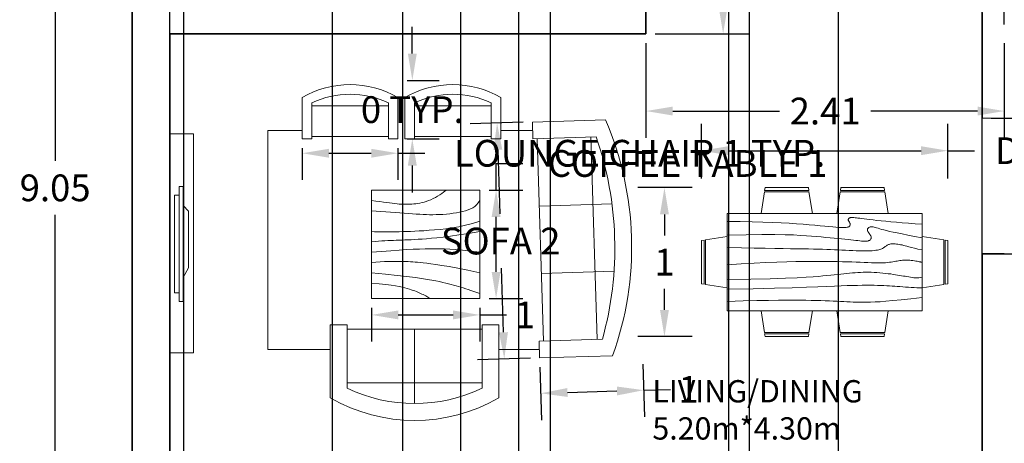
# Model space of a CAD drawing. Units: metres. Extents: x 1988.6 to 2001.1, y 2192 to 2202.5.
# Tile 2 of 6: x 1988.6 to 1995.3, y 2195.5 to 2198.4. Entities that reach past the tile are written whole.
import ezdxf

# ---------------------------------------------------------------- set-up
doc = ezdxf.new("R2010")
doc.units = ezdxf.units.M
for name, color, linetype, lineweight in [('A-ANNO-DIMS', 2, 'Continuous', 18), ('A-AREA-IDEN', 7, 'Continuous', 18), ('A-EQPM', 8, 'Continuous', 13), ('A-FURN', 9, 'Continuous', 15), ('A-WALL', 7, 'Continuous', 35)]:
    doc.layers.add(name, color=color, linetype=linetype, lineweight=lineweight)
doc.styles.get("Standard").update_dxf_attribs({"font": 'arial.ttf'})
doc.dimstyles.get("Standard").update_dxf_attribs({"dimtxt": 0.18, "dimasz": 0.18, "dimexe": 0.18, "dimexo": 0.0625, "dimgap": 0.09, "dimtad": 0, "dimtih": 1, "dimtoh": 1, "dimdec": 4, "dimzin": 0, "dimdsep": 46, "dimtxsty": 'Standard', "dimcen": 0.09, "dimadec": 0, "dimazin": 0, "dimtfac": 1, "dimtdec": 4, "dimtofl": 0, "dimtmove": 0, "dimatfit": 3, "dimfxl": 1, "dimtolj": 1, "dimtzin": 0, "dimarcsym": 0})

# ---------------------------------------------------------------- blocks, each defined once
blk = doc.blocks.new('Dining Set - 36 x 72 in.')
for p, q in [((-22.2343, 26.00059), (-23.4847, 17.99762)), ((-22.2304, 26), (-5.7608, 26)), ((-22, 27.5), (-22.1562, 26.50042)), ((-5.8416, 26.5), (-22.1534, 26.5)), ((-22, 27.5), (-6, 27.5)), ((-5.8437, 26.49966), (-6, 27.5)), ((-4.5152, 17.99762), (-5.7655, 25.99926)), ((5.7657, 26.00059), (4.5153, 17.99762)), ((5.7696, 26), (22.2392, 26)), ((6, 27.5), (5.8438, 26.50042)), ((22.1584, 26.5), (5.8466, 26.5)), ((6, 27.5), (22, 27.5)), ((22.1563, 26.49966), (22, 27.5)), ((23.4848, 17.99762), (22.2345, 25.99926)), ((36, 18), (-36, 18)), ((-36, 18), (-36, -18)), ((36, -18), (36, 18)), ((-45.5, 8), (-44.5004, 8.15617)), ((-45.5, 8), (-45.5, -8)), ((-44.5, -8.15843), (-44.5, 8.15338)), ((-44.0006, 8.23428), (-35.9976, 9.48474)), ((-44, 8.23041), (-44, -8.23915)), ((44.0006, 8.23428), (35.9976, 9.48474)), ((44, 8.23041), (44, -8.23915)), ((44.5, -8.15843), (44.5, 8.15338)), ((45.5, 8), (44.5005, 8.15617)), ((45.5, 8), (45.5, -8)), ((-44.4997, -8.15631), (-45.5, -8)), ((-35.9976, -9.48476), (-43.9993, -8.2345)), ((35.9976, -9.48476), (43.9993, -8.2345)), ((44.4997, -8.15631), (45.5, -8)), ((-36, -18), (36, -18)), ((-22.2343, -26.0006), (-23.4847, -17.99762)), ((-4.5152, -17.99762), (-5.7655, -25.99928)), ((5.7657, -26.0006), (4.5153, -17.99762)), ((23.4848, -17.99762), (22.2345, -25.99928)), ((-22.2304, -26), (-5.7608, -26)), ((-22, -27.5), (-22.1562, -26.50044)), ((-5.8416, -26.5), (-22.1534, -26.5)), ((-22, -27.5), (-6, -27.5)), ((-5.8437, -26.49967), (-6, -27.5)), ((5.7696, -26), (22.2392, -26)), ((6, -27.5), (5.8438, -26.50044)), ((22.1584, -26.5), (5.8466, -26.5)), ((6, -27.5), (22, -27.5)), ((22.1563, -26.49967), (22, -27.5))]:
    blk.add_line(p, q)
for points in [[(-36, 15), (-31.1772, 14.97754), (-26.8079, 14.91406), (-22.8538, 14.81543), (-19.276, 14.6875), (-16.0362, 14.53613), (-13.0957, 14.36718), (-10.4159, 14.18652), (-7.9583, 14), (-5.6904, 13.81315), (-3.6035, 13.63021), (-1.6954, 13.45508), (0.0365, 13.29166), (1.5945, 13.14388), (2.9811, 13.01562), (4.1988, 12.9108), (5.25, 12.83333), (6.1393, 12.78613), (6.8802, 12.76823), (7.4883, 12.77767), (7.9792, 12.8125), (8.3685, 12.87077), (8.6719, 12.95052), (8.9049, 13.0498), (9.0833, 13.16666), (9.2205, 13.29899), (9.3216, 13.44401), (9.3895, 13.59879), (9.4271, 13.76041), (9.4373, 13.92594), (9.4232, 14.09245), (9.3875, 14.257), (9.3333, 14.41666), (9.2638, 14.56917), (9.1836, 14.71484), (9.0975, 14.85465), (9.0104, 14.98958), (8.9272, 15.1206), (8.8529, 15.2487), (8.7922, 15.37483), (8.75, 15.5), (8.7305, 15.62467), (8.7344, 15.74739), (8.7617, 15.86621), (8.8125, 15.97916), (8.8867, 16.08431), (8.9844, 16.17968), (9.1055, 16.26334), (9.25, 16.33333), (9.4189, 16.38802), (9.6172, 16.42708), (9.8506, 16.45052), (10.125, 16.45833), (10.4463, 16.45052), (10.8203, 16.42708), (11.2529, 16.38802), (11.75, 16.33333), (12.3184, 16.26318), (12.9694, 16.17838), (13.7151, 16.07991), (14.5677, 15.96875), (15.5395, 15.84586), (16.6426, 15.71224), (17.8893, 15.56884), (19.2917, 15.41666), (20.859, 15.25667), (22.5879, 15.08984), (24.4721, 14.91715), (26.5052, 14.73958), (28.6809, 14.5581), (30.9929, 14.3737), (33.4347, 14.18733), (36, 14)], [(-36, 10), (-28.9766, 10.14274), (-23.1725, 10.20442), (-18.4241, 10.19775), (-14.5677, 10.13541), (-11.4399, 10.03011), (-8.877, 9.89453), (-6.7154, 9.74137), (-4.7917, 9.58333), (-2.9698, 9.43082), (-1.2246, 9.28515), (0.4415, 9.14534), (2.026, 9.01041), (3.5266, 8.87939), (4.9408, 8.7513), (6.266, 8.62516), (7.5, 8.5), (8.6411, 8.37549), (9.6914, 8.2539), (10.6538, 8.13818), (11.5312, 8.03125), (12.3267, 7.93603), (13.043, 7.85547), (13.6831, 7.79248), (14.25, 7.75), (14.7471, 7.7303), (15.1797, 7.73307), (15.5537, 7.75732), (15.875, 7.80208), (16.1494, 7.86637), (16.3828, 7.94922), (16.5811, 8.04964), (16.75, 8.16666), (16.8944, 8.29915), (17.0143, 8.44531), (17.1089, 8.60319), (17.1771, 8.77083), (17.218, 8.94629), (17.2305, 9.1276), (17.2137, 9.31282), (17.1667, 9.5), (17.0895, 9.6875), (16.987, 9.875), (16.8649, 10.0625), (16.7292, 10.25), (16.5856, 10.4375), (16.4401, 10.625), (16.2985, 10.8125), (16.1667, 11), (16.05, 11.18733), (15.9518, 11.3737), (15.8752, 11.5581), (15.8229, 11.73958), (15.798, 11.91715), (15.8034, 12.08984), (15.842, 12.25667), (15.9167, 12.41666), (16.0295, 12.56836), (16.1784, 12.70833), (16.3605, 12.83268), (16.5729, 12.9375), (16.8127, 13.01888), (17.0768, 13.07291), (17.3625, 13.0957), (17.6667, 13.08333), (17.9894, 13.03312), (18.3418, 12.94726), (18.7382, 12.82918), (19.1927, 12.68229), (19.7195, 12.51001), (20.3327, 12.31575), (21.0465, 12.10294), (21.875, 11.875), (22.8357, 11.63354), (23.959, 11.37304), (25.2786, 11.08618), (26.8282, 10.76562), (28.6414, 10.40405), (30.752, 9.99414), (33.1936, 9.52856), (36, 9)], [(-36, 5.5), (-30.7157, 5.3348), (-26.069, 5.20963), (-21.9946, 5.11767), (-18.4271, 5.05208), (-15.3009, 5.00602), (-12.5508, 4.97265), (-10.1112, 4.94515), (-7.9167, 4.91666), (-5.909, 4.88167), (-4.0586, 4.83984), (-2.3429, 4.79215), (-0.7396, 4.73958), (0.7739, 4.6831), (2.22, 4.6237), (3.6213, 4.56233), (5, 4.5), (6.373, 4.43782), (7.7344, 4.3776), (9.0723, 4.32129), (10.375, 4.27083), (11.6309, 4.22819), (12.8281, 4.19531), (13.9551, 4.17415), (15, 4.16666), (15.954, 4.17448), (16.819, 4.19791), (17.6001, 4.23698), (18.3021, 4.29166), (18.9299, 4.36198), (19.4883, 4.44791), (19.9823, 4.54948), (20.4167, 4.66666), (20.7969, 4.79899), (21.1302, 4.94401), (21.4245, 5.09879), (21.6875, 5.26041), (21.9271, 5.42594), (22.1511, 5.59245), (22.3672, 5.757), (22.5834, 5.91666), (22.8065, 6.06868), (23.0404, 6.21093), (23.2879, 6.34147), (23.5521, 6.45833), (23.8358, 6.55957), (24.142, 6.64323), (24.4735, 6.70735), (24.8334, 6.75), (25.2235, 6.76969), (25.642, 6.76692), (26.0858, 6.74267), (26.5521, 6.69791), (27.0379, 6.63362), (27.5404, 6.55078), (28.0565, 6.45036), (28.5834, 6.33333), (29.1242, 6.19987), (29.7071, 6.04687), (30.3661, 5.87044), (31.1354, 5.66666), (32.0493, 5.43164), (33.142, 5.16146), (34.4475, 4.85221), (36, 4.5)], [(-36, -1), (-30.7915, -0.6591), (-26.0195, -0.38216), (-21.6519, -0.16284), (-17.6563, 0.00521), (-14.0005, 0.12833), (-10.6523, 0.21289), (-7.5796, 0.26522), (-4.75, 0.29166), (-2.134, 0.29793), (0.2878, 0.28711), (2.5317, 0.26163), (4.6146, 0.22396), (6.5529, 0.17651), (8.3633, 0.12174), (10.0623, 0.06209), (11.6667, 0), (13.1899, -0.06201), (14.6341, -0.1211), (15.9982, -0.17432), (17.2813, -0.21875), (18.4823, -0.25147), (19.6003, -0.26953), (20.6343, -0.27002), (21.5834, -0.25), (22.4481, -0.20768), (23.2357, -0.14584), (23.9549, -0.06836), (24.6146, 0.02083), (25.2235, 0.11784), (25.7904, 0.21875), (26.3241, 0.31966), (26.8334, 0.41666), (27.3265, 0.50618), (27.8099, 0.58593), (28.2894, 0.65397), (28.7709, 0.70833), (29.2601, 0.74707), (29.763, 0.76823), (30.2855, 0.76985), (30.8334, 0.75), (31.4088, 0.70784), (31.9994, 0.64713), (32.589, 0.57275), (33.1615, 0.48958), (33.7008, 0.4025), (34.1908, 0.3164), (34.6153, 0.23616), (34.9584, 0.16666), (35.2099, 0.11165), (35.3848, 0.07031), (35.504, 0.04069), (35.5886, 0.02083), (35.6594, 0.00879), (35.7377, 0.0026), (35.8442, 0.00032), (36, 0)], [(-36, -6.5), (-27.1843, -6.31267), (-20.084, -6.1263), (-14.469, -5.9419), (-10.1094, -5.76042), (-6.7752, -5.58285), (-4.2363, -5.41016), (-2.2629, -5.24333), (-0.625, -5.08334), (0.8708, -4.93099), (2.2715, -4.78646), (3.5872, -4.64974), (4.8281, -4.52084), (6.0046, -4.39974), (7.127, -4.28646), (8.2053, -4.18099), (9.25, -4.08334), (10.2705, -3.99382), (11.2734, -3.91407), (12.2647, -3.84603), (13.25, -3.79167), (14.2354, -3.75293), (15.2266, -3.73177), (16.2295, -3.73015), (17.25, -3.75), (18.2912, -3.79248), (19.3451, -3.85547), (20.4009, -3.93604), (21.4479, -4.03125), (22.4754, -4.13819), (23.4727, -4.25391), (24.4289, -4.37549), (25.3334, -4.5), (26.1785, -4.62492), (26.9694, -4.74935), (27.7145, -4.87281), (28.4219, -4.99479), (29.1, -5.11483), (29.7572, -5.23242), (30.4016, -5.34709), (31.0417, -5.45834), (31.6837, -5.56437), (32.3262, -5.65821), (32.9658, -5.73153), (33.599, -5.77604), (34.2224, -5.78345), (34.8327, -5.74545), (35.4264, -5.65373), (36, -5.5)], [(-36, -10), (-26.4022, -9.81299), (-18.4675, -9.62891), (-11.9839, -9.45069), (-6.7396, -9.28125), (-2.5226, -9.12354), (0.8789, -8.98047), (3.6769, -8.85498), (6.0833, -8.75), (8.2767, -8.66765), (10.3021, -8.60677), (12.1712, -8.56543), (13.8958, -8.54167), (15.4876, -8.53353), (16.9583, -8.53907), (18.3197, -8.55632), (19.5834, -8.58334), (20.7616, -8.61841), (21.8685, -8.66081), (22.9188, -8.71004), (23.9271, -8.76563), (24.9081, -8.82707), (25.8763, -8.89388), (26.8465, -8.96558), (27.8334, -9.04167), (28.8474, -9.12118), (29.8828, -9.20117), (30.93, -9.27824), (31.9792, -9.34896), (33.0205, -9.40991), (34.0443, -9.45768), (35.0407, -9.48885), (36, -9.5)], [(-36, -14.5), (-30.0881, -14.33513), (-25.0332, -14.21224), (-20.7312, -14.12647), (-17.0781, -14.07292), (-13.97, -14.04671), (-11.3027, -14.04297), (-8.9724, -14.05681), (-6.875, -14.08334), (-4.9224, -14.11833), (-3.0905, -14.16016), (-1.3709, -14.20785), (0.2448, -14.26042), (1.7647, -14.3169), (3.1973, -14.3763), (4.5507, -14.43767), (5.8333, -14.5), (7.0554, -14.5621), (8.235, -14.62175), (9.3922, -14.67652), (10.5469, -14.72396), (11.7192, -14.76164), (12.929, -14.78711), (14.1965, -14.79794), (15.5417, -14.79167), (16.9933, -14.76424), (18.6152, -14.70508), (20.4804, -14.60197), (22.6615, -14.44271), (25.2312, -14.21509), (28.2624, -13.9069), (31.8277, -13.50594), (36, -13)]]:
    blk.add_lwpolyline(points)
blk = doc.blocks.new('Table - Square Woodgrain 42 x 42 in.')
blk.add_line((0, -42), (42, -42))
for points in [[(0, -4), (1.704, -4.2172), (3.2358, -4.4188), (4.615, -4.604), (5.8615, -4.7721), (6.9951, -4.9224), (8.0357, -5.0541), (9.0031, -5.1667), (9.9171, -5.2594), (10.7951, -5.3316), (11.6445, -5.3836), (12.4702, -5.4157), (13.277, -5.4283), (14.0698, -5.4217), (14.8535, -5.3964), (15.6331, -5.3526), (16.4133, -5.2908), (17.1986, -5.2103), (17.9913, -5.1062), (18.793, -4.9727), (19.6056, -4.8038), (20.4307, -4.5937), (21.2701, -4.3365), (22.1256, -4.0262), (22.9989, -3.6571), (23.888, -3.2272), (24.7756, -2.7516), (25.6408, -2.2491), (26.4624, -1.7387), (27.2195, -1.2395), (27.891, -0.7703), (28.456, -0.3501), (28.8934, 0.002)], [(0, -42), (0, 0), (42, 0), (42, -42)], [(0, -8), (1.8203, -8.1001), (3.6741, -8.2149), (5.5411, -8.3408), (7.4011, -8.4741), (9.2339, -8.6112), (11.0193, -8.7484), (12.7371, -8.8821), (14.3671, -9.0086), (15.8954, -9.1246), (17.3337, -9.2278), (18.6997, -9.3159), (20.0116, -9.387), (21.2871, -9.4389), (22.5442, -9.4696), (23.8008, -9.477), (25.0749, -9.459), (26.3791, -9.4137), (27.7049, -9.3403), (29.0383, -9.2382), (30.3655, -9.1068), (31.6728, -8.9455), (32.9461, -8.7535), (34.1717, -8.5304), (35.3358, -8.2756), (36.4268, -7.9863), (37.443, -7.6521), (38.3849, -7.2603), (39.253, -6.7986), (40.048, -6.2542), (40.7705, -5.6147), (41.421, -4.8674), (42, -4)], [(42, -12), (39.1784, -12.8621), (36.4519, -13.5654), (33.8246, -14.1294), (31.3004, -14.5731), (28.8832, -14.9161), (26.577, -15.1775), (24.3858, -15.3768), (22.3136, -15.5332), (20.3622, -15.6632), (18.5254, -15.7718), (16.7947, -15.8612), (15.1618, -15.9338), (13.6183, -15.9916), (12.1558, -16.0369), (10.7659, -16.0718), (9.4403, -16.0987), (8.1703, -16.1191), (6.9461, -16.1325), (5.7577, -16.1377), (4.595, -16.1335), (3.4479, -16.1188), (2.3064, -16.0924), (1.1604, -16.0532), (0, -16)], [(42, -16), (37.6529, -16.7365), (33.8802, -17.329), (30.6179, -17.7961), (27.8015, -18.1561), (25.3668, -18.4275), (23.2497, -18.6288), (21.3859, -18.7785), (19.7111, -18.8949), (18.1693, -18.9939), (16.7375, -19.0795), (15.401, -19.1534), (14.1449, -19.217), (12.9544, -19.2717), (11.8148, -19.3191), (10.7113, -19.3606), (9.6291, -19.3976), (8.5534, -19.4323), (7.47, -19.4689), (6.3643, -19.5122), (5.222, -19.5672), (4.0288, -19.6386), (2.7703, -19.7313), (1.4321, -19.8501), (0, -20)], [(0, -24), (3.9243, -23.6805), (7.4766, -23.4138), (10.6891, -23.1954), (13.5943, -23.0205), (16.2247, -22.8847), (18.6125, -22.7832), (20.7903, -22.7116), (22.7903, -22.6651), (24.6563, -22.642), (26.4764, -22.6507), (28.35, -22.7024), (30.3766, -22.8084), (32.6555, -22.98), (35.2861, -23.2283), (38.3678, -23.5645), (42, -24)], [(42, -32), (37.392, -31.017), (33.4585, -30.2231), (30.1291, -29.5949), (27.3334, -29.109), (25.0009, -28.742), (23.0612, -28.4707), (21.4439, -28.2716), (20.0786, -28.1215), (18.8998, -28.0002), (17.8609, -27.9014), (16.9206, -27.8219), (16.0371, -27.7588), (15.1691, -27.709), (14.2748, -27.6693), (13.3128, -27.6368), (12.2415, -27.6083), (11.0295, -27.5824), (9.6867, -27.5643), (8.233, -27.5608), (6.6884, -27.5787), (5.0728, -27.6248), (3.4062, -27.7058), (1.7086, -27.8286), (0, -28)], [(0, -32), (5.4026, -32.5358), (9.9494, -33.019), (13.7424, -33.4553), (16.8834, -33.8505), (19.4743, -34.2106), (21.6171, -34.5413), (23.4136, -34.8486), (24.9657, -35.1382), (26.3614, -35.4156), (27.6332, -35.6841), (28.7995, -35.9467), (29.8788, -36.2064), (30.8897, -36.4661), (31.8507, -36.7288), (32.7802, -36.9973), (33.6968, -37.2747), (34.6175, -37.5635), (35.5531, -37.8651), (36.5128, -38.1805), (37.506, -38.5108), (38.5421, -38.8568), (39.6302, -39.2197), (40.7797, -39.6004), (42, -40)], [(0, -36), (3.0098, -36.2857), (5.5354, -36.5643), (7.6368, -36.8359), (9.374, -37.1009), (10.807, -37.3597), (11.9957, -37.6126), (13.0002, -37.8599), (13.8804, -38.102), (14.6874, -38.3393), (15.4365, -38.5729), (16.1338, -38.8041), (16.7858, -39.0341), (17.3987, -39.264), (17.9787, -39.4952), (18.5322, -39.7288), (19.0655, -39.9662), (19.5832, -40.2081), (20.0842, -40.4544), (20.5657, -40.7046), (21.0249, -40.9581), (21.459, -41.2144), (21.8653, -41.4731), (22.2409, -41.7335), (22.5831, -41.9951)]]:
    blk.add_lwpolyline(points)
blk = doc.blocks.new('Sofa - Roundback 7 ft.')
for p, q in [((-12.00002, -32.4421), (-12.00003, -6.5971)), ((11.99997, -32.4421), (11.99998, -6.5971)), ((-36.000027, -34), (-36.000027, -11.4696)), ((-35.999844, -13.3819), (35.9998, -13.3819)), ((35.99998, -34), (35.99998, -11.4696)), ((-36.000027, -32.4421), (35.99998, -32.4421))]:
    blk.add_line(p, q)
for points in [[(-36.000027, -34), (-42.000027, -34), (-42.000027, -8)], [(41.99998, -8), (41.99998, -34), (35.99998, -34)]]:
    blk.add_lwpolyline(points)
for centre, radius, start, end in [((0, -114.25), 114.25, 68.43141, 111.5686), ((-0.00001, -127.1968), 121.1968, 72.72033, 107.2797)]:
    blk.add_arc(centre, radius, start, end)
blk = doc.blocks.new('LOUNGE-CHAIR')
for p, q in [((0.0643, 0.0004), (0.0643, 0.2424)), ((0.0643, 0.2219), (0.5798, 0.2219)), ((0.5798, 0.0004), (0.5798, 0.2424)), ((0.0643, 0.0172), (0.5798, 0.0172))]:
    blk.add_line(p, q)
for points in [[(0.0643, 0.0004), (-0.0002, 0.0004), (-0.0002, 0.2797)], [(0.6442, 0.2797), (0.6442, 0.0004), (0.5798, 0.0004)]]:
    blk.add_lwpolyline(points)
for centre, radius, start, end in [((0.322, -0.2815), 0.6471, 60.13715, 119.8628), ((0.322, -0.2937), 0.5948, 64.32083, 115.6792)]:
    blk.add_arc(centre, radius, start, end)
blk = doc.blocks.new('*D40')
at = {"layer": 'A-ANNO-DIMS', "color": 0, "lineweight": -2, "transparency": 16777216}
for p, q in [((1990.5252, 2197.4959), (1990.5252, 2197.2818)), ((1991.1696, 2197.4959), (1991.1696, 2197.2818)), ((1990.7052, 2197.4618), (1990.9896, 2197.4618)), ((1991.1696, 2197.4618), (1991.3496, 2197.4618))]:
    blk.add_line(p, q, dxfattribs=at)
at = {"layer": 'A-ANNO-DIMS', "color": 0, "transparency": 16777216}
for points in [[(1990.7052, 2197.4918), (1990.7052, 2197.4318), (1990.5252, 2197.4618)], [(1990.9896, 2197.4918), (1990.9896, 2197.4318), (1991.1696, 2197.4618)]]:
    blk.add_solid(points, dxfattribs=at)
at = {"layer": 'Defpoints', "color": 0, "transparency": 16777216}
for p in [(1990.5252, 2197.5584), (1991.1696, 2197.5584), (1991.1696, 2197.4618)]:
    blk.add_point(p, dxfattribs=at)
at = {"layer": 'A-ANNO-DIMS', "color": 0, "transparency": 16777216, "insert": (1992.7958, 2197.4618), "char_height": 0.18, "attachment_point": 5}
blk.add_mtext('\\A1;LOUNGE CHAIR 1 TYP.', dxfattribs=at)
blk = doc.blocks.new('*D41')
at = {"layer": 'A-ANNO-DIMS', "color": 0, "lineweight": -2, "transparency": 16777216}
for p, q in [((1991.2663, 2198.1322), (1991.2663, 2198.3122)), ((1991.2321, 2197.9522), (1991.4463, 2197.9522)), ((1991.2321, 2197.5584), (1991.4463, 2197.5584)), ((1991.2663, 2197.3784), (1991.2663, 2197.1984))]:
    blk.add_line(p, q, dxfattribs=at)
at = {"layer": 'A-ANNO-DIMS', "color": 0, "transparency": 16777216}
for points in [[(1991.2363, 2198.1322), (1991.2963, 2198.1322), (1991.2663, 2197.9522)], [(1991.2363, 2197.3784), (1991.2963, 2197.3784), (1991.2663, 2197.5584)]]:
    blk.add_solid(points, dxfattribs=at)
at = {"layer": 'Defpoints', "color": 0, "transparency": 16777216}
for p in [(1991.1696, 2197.9522), (1991.2663, 2197.9522), (1991.1696, 2197.5584)]:
    blk.add_point(p, dxfattribs=at)
at = {"layer": 'A-ANNO-DIMS', "color": 0, "transparency": 16777216, "insert": (1991.2663, 2197.7553), "char_height": 0.18, "attachment_point": 5}
blk.add_mtext('\\A1;0 TYP.', dxfattribs=at)
blk = doc.blocks.new('*D46')
at = {"layer": 'A-ANNO-DIMS', "color": 0, "lineweight": -2, "transparency": 16777216}
for p, q in [((1993.2119, 2197.2927), (1993.2119, 2197.659)), ((1994.8706, 2197.2927), (1994.8706, 2197.659)), ((1993.3919, 2197.479), (1994.6906, 2197.479)), ((1994.8706, 2197.479), (1995.0506, 2197.479))]:
    blk.add_line(p, q, dxfattribs=at)
at = {"layer": 'A-ANNO-DIMS', "color": 0, "transparency": 16777216}
for points in [[(1993.3919, 2197.509), (1993.3919, 2197.449), (1993.2119, 2197.479)], [(1994.6906, 2197.509), (1994.6906, 2197.449), (1994.8706, 2197.479)]]:
    blk.add_solid(points, dxfattribs=at)
at = {"layer": 'Defpoints', "color": 0, "transparency": 16777216}
for p in [(1994.8706, 2197.479), (1993.2119, 2197.2302), (1994.8706, 2197.2302)]:
    blk.add_point(p, dxfattribs=at)
at = {"layer": 'A-ANNO-DIMS', "color": 0, "transparency": 16777216, "insert": (1995.9486, 2197.479), "char_height": 0.18, "attachment_point": 5}
blk.add_mtext('\\A1;DINING SET 2', dxfattribs=at)
blk = doc.blocks.new('*D47')
at = {"layer": 'A-ANNO-DIMS', "color": 0, "lineweight": -2, "transparency": 16777216}
for p, q in [((1993.1494, 2197.2302), (1992.7831, 2197.2302)), ((1992.9631, 2197.0502), (1992.9631, 2196.9093)), ((1992.9631, 2196.4076), (1992.9631, 2196.5485)), ((1993.1494, 2196.2276), (1992.7831, 2196.2276))]:
    blk.add_line(p, q, dxfattribs=at)
at = {"layer": 'A-ANNO-DIMS', "color": 0, "transparency": 16777216}
for points in [[(1992.9331, 2197.0502), (1992.9931, 2197.0502), (1992.9631, 2197.2302)], [(1992.9331, 2196.4076), (1992.9931, 2196.4076), (1992.9631, 2196.2276)]]:
    blk.add_solid(points, dxfattribs=at)
at = {"layer": 'Defpoints', "color": 0, "transparency": 16777216}
for p in [(1992.9631, 2197.2302), (1993.2119, 2197.2302), (1993.2119, 2196.2276)]:
    blk.add_point(p, dxfattribs=at)
at = {"layer": 'A-ANNO-DIMS', "color": 0, "transparency": 16777216, "insert": (1992.9631, 2196.7289), "char_height": 0.18, "attachment_point": 5}
blk.add_mtext('\\A1;1', dxfattribs=at)
blk = doc.blocks.new('*D48')
at = {"layer": 'A-ANNO-DIMS', "color": 0, "lineweight": -2, "transparency": 16777216}
for p, q in [((1991.8301, 2197.2128), (1991.8301, 2197.3928)), ((1991.8301, 2197.3928), (1992.0101, 2197.3928)), ((1991.7832, 2197.2128), (1992.0101, 2197.2128)), ((1991.8301, 2196.6633), (1991.8301, 2197.0328)), ((1991.7832, 2196.4833), (1992.0101, 2196.4833))]:
    blk.add_line(p, q, dxfattribs=at)
at = {"layer": 'A-ANNO-DIMS', "color": 0, "transparency": 16777216}
for points in [[(1991.8001, 2197.0328), (1991.8601, 2197.0328), (1991.8301, 2197.2128)], [(1991.8001, 2196.6633), (1991.8601, 2196.6633), (1991.8301, 2196.4833)]]:
    blk.add_solid(points, dxfattribs=at)
at = {"layer": 'Defpoints', "color": 0, "transparency": 16777216}
for p in [(1991.7207, 2197.2128), (1991.8301, 2197.2128), (1991.7207, 2196.4833)]:
    blk.add_point(p, dxfattribs=at)
at = {"layer": 'A-ANNO-DIMS', "color": 0, "transparency": 16777216, "insert": (1993.1188, 2197.3928), "char_height": 0.18, "attachment_point": 5}
blk.add_mtext('\\A1;COFFEE TABLE 1', dxfattribs=at)
blk = doc.blocks.new('*D49')
at = {"layer": 'A-ANNO-DIMS', "color": 0, "lineweight": -2, "transparency": 16777216}
for p, q in [((1990.9912, 2196.4208), (1990.9912, 2196.1939)), ((1991.1712, 2196.3739), (1991.5407, 2196.3739)), ((1991.7207, 2196.4208), (1991.7207, 2196.1939)), ((1991.7207, 2196.3739), (1991.9007, 2196.3739))]:
    blk.add_line(p, q, dxfattribs=at)
at = {"layer": 'A-ANNO-DIMS', "color": 0, "transparency": 16777216}
for points in [[(1991.1712, 2196.4039), (1991.1712, 2196.3439), (1990.9912, 2196.3739)], [(1991.5407, 2196.4039), (1991.5407, 2196.3439), (1991.7207, 2196.3739)]]:
    blk.add_solid(points, dxfattribs=at)
at = {"layer": 'Defpoints', "color": 0, "transparency": 16777216}
for p in [(1990.9912, 2196.4833), (1991.7207, 2196.4833), (1991.7207, 2196.3739)]:
    blk.add_point(p, dxfattribs=at)
at = {"layer": 'A-ANNO-DIMS', "color": 0, "transparency": 16777216, "insert": (1992.0239, 2196.3739), "char_height": 0.18, "attachment_point": 5}
blk.add_mtext('\\A1;1', dxfattribs=at)
blk = doc.blocks.new('*D50')
at = {"layer": 'A-ANNO-DIMS', "color": 0, "lineweight": -2, "transparency": 16777216}
for p, q in [((1992.0123, 2197.67), (1991.6567, 2197.6591)), ((1991.8421, 2197.4847), (1991.8553, 2197.0539)), ((1991.8797, 2196.257), (1991.8665, 2196.6877)), ((1992.0609, 2196.0824), (1991.7053, 2196.0715))]:
    blk.add_line(p, q, dxfattribs=at)
at = {"layer": 'A-ANNO-DIMS', "color": 0, "transparency": 16777216}
for points in [[(1991.8721, 2197.4856), (1991.8121, 2197.4838), (1991.8366, 2197.6646)], [(1991.9097, 2196.2579), (1991.8497, 2196.256), (1991.8852, 2196.077)]]:
    blk.add_solid(points, dxfattribs=at)
at = {"layer": 'Defpoints', "color": 0, "transparency": 16777216}
for p in [(1992.0747, 2197.6719), (1991.8852, 2196.077), (1992.1233, 2196.0843)]:
    blk.add_point(p, dxfattribs=at)
at = {"layer": 'A-ANNO-DIMS', "color": 0, "transparency": 16777216, "insert": (1991.8609, 2196.8708), "char_height": 0.18, "attachment_point": 5}
blk.add_mtext('\\A1;SOFA 2', dxfattribs=at)
blk = doc.blocks.new('*D51')
at = {"layer": 'A-ANNO-DIMS', "color": 0, "lineweight": -2, "transparency": 16777216}
for p, q in [((1992.8182, 2196.0431), (1992.8291, 2195.6875)), ((1992.1252, 2196.0219), (1992.1361, 2195.6663)), ((1992.3105, 2195.8517), (1992.6437, 2195.8619)), ((1992.8236, 2195.8674), (1993.0035, 2195.8729))]:
    blk.add_line(p, q, dxfattribs=at)
at = {"layer": 'A-ANNO-DIMS', "color": 0, "transparency": 16777216}
for points in [[(1992.3096, 2195.8817), (1992.3115, 2195.8217), (1992.1306, 2195.8462)], [(1992.6428, 2195.8919), (1992.6446, 2195.8319), (1992.8236, 2195.8674)]]:
    blk.add_solid(points, dxfattribs=at)
at = {"layer": 'Defpoints', "color": 0, "transparency": 16777216}
for p in [(1992.8163, 2196.1055), (1992.1233, 2196.0843), (1992.8236, 2195.8674)]:
    blk.add_point(p, dxfattribs=at)
at = {"layer": 'A-ANNO-DIMS', "color": 0, "transparency": 16777216, "insert": (1993.1267, 2195.8729), "char_height": 0.18, "attachment_point": 5}
blk.add_mtext('\\A1;1', dxfattribs=at)
blk = doc.blocks.new('*D53')
at = {"layer": 'A-ANNO-DIMS', "color": 0, "lineweight": -2, "transparency": 16777216}
for p, q in [((1989.3193, 2201.7538), (1988.6823, 2201.7538)), ((1988.8623, 2201.5738), (1988.8623, 2197.4107)), ((1988.8623, 2192.8838), (1988.8623, 2197.0469)), ((1989.3193, 2192.7038), (1988.6823, 2192.7038))]:
    blk.add_line(p, q, dxfattribs=at)
at = {"layer": 'A-ANNO-DIMS', "color": 0, "transparency": 16777216}
for points in [[(1988.8323, 2201.5738), (1988.8923, 2201.5738), (1988.8623, 2201.7538)], [(1988.8323, 2192.8838), (1988.8923, 2192.8838), (1988.8623, 2192.7038)]]:
    blk.add_solid(points, dxfattribs=at)
at = {"layer": 'Defpoints', "color": 0, "transparency": 16777216}
for p in [(1988.8623, 2201.7538), (1989.3818, 2201.7538), (1989.3818, 2192.7038)]:
    blk.add_point(p, dxfattribs=at)
at = {"layer": 'A-ANNO-DIMS', "color": 0, "transparency": 16777216, "insert": (1988.8623, 2197.2288), "char_height": 0.18, "attachment_point": 5}
blk.add_mtext('\\A1;9.05', dxfattribs=at)
blk = doc.blocks.new('*D59')
at = {"layer": 'A-ANNO-DIMS', "color": 0, "lineweight": -2, "transparency": 16777216}
for p, q in [((1989.7282, 2194.023), (1989.7282, 2202.4533)), ((1990.7282, 2193.0163), (1990.7282, 2202.4533)), ((1989.9082, 2202.2733), (1990.1051, 2202.2733)), ((1990.5482, 2202.2733), (1990.3514, 2202.2733))]:
    blk.add_line(p, q, dxfattribs=at)
at = {"layer": 'A-ANNO-DIMS', "color": 0, "transparency": 16777216}
for points in [[(1989.9082, 2202.3033), (1989.9082, 2202.2433), (1989.7282, 2202.2733)], [(1990.5482, 2202.3033), (1990.5482, 2202.2433), (1990.7282, 2202.2733)]]:
    blk.add_solid(points, dxfattribs=at)
at = {"layer": 'Defpoints', "color": 0, "transparency": 16777216}
for p in [(1990.7282, 2202.2733), (1989.7282, 2193.9605), (1990.7282, 2192.9538)]:
    blk.add_point(p, dxfattribs=at)
at = {"layer": 'A-ANNO-DIMS', "color": 0, "transparency": 16777216, "insert": (1990.2282, 2202.2733), "char_height": 0.18, "attachment_point": 5}
blk.add_mtext('\\A1;1', dxfattribs=at)
blk = doc.blocks.new('*D60')
at = {"layer": 'A-ANNO-DIMS', "color": 0, "lineweight": -2, "transparency": 16777216}
for p, q in [((1990.7282, 2193.0163), (1990.7282, 2202.4533)), ((1992.1958, 2193.0163), (1992.1958, 2202.4533)), ((1990.9082, 2202.2733), (1991.1467, 2202.2733)), ((1992.0158, 2202.2733), (1991.7773, 2202.2733))]:
    blk.add_line(p, q, dxfattribs=at)
at = {"layer": 'A-ANNO-DIMS', "color": 0, "transparency": 16777216}
for points in [[(1990.9082, 2202.3033), (1990.9082, 2202.2433), (1990.7282, 2202.2733)], [(1992.0158, 2202.3033), (1992.0158, 2202.2433), (1992.1958, 2202.2733)]]:
    blk.add_solid(points, dxfattribs=at)
at = {"layer": 'Defpoints', "color": 0, "transparency": 16777216}
for p in [(1992.1958, 2202.2733), (1990.7282, 2192.9538), (1992.1958, 2192.9538)]:
    blk.add_point(p, dxfattribs=at)
at = {"layer": 'A-ANNO-DIMS', "color": 0, "transparency": 16777216, "insert": (1991.462, 2202.2733), "char_height": 0.18, "attachment_point": 5}
blk.add_mtext('\\A1;1.47', dxfattribs=at)
blk = doc.blocks.new('*D61')
at = {"layer": 'A-ANNO-DIMS', "color": 0, "lineweight": -2, "transparency": 16777216}
for p, q in [((1992.1958, 2193.0163), (1992.1958, 2202.4533)), ((1993.3958, 2193.0163), (1993.3958, 2202.4533)), ((1992.3758, 2202.2733), (1992.5513, 2202.2733)), ((1993.2158, 2202.2733), (1993.0402, 2202.2733))]:
    blk.add_line(p, q, dxfattribs=at)
at = {"layer": 'A-ANNO-DIMS', "color": 0, "transparency": 16777216}
for points in [[(1992.3758, 2202.3033), (1992.3758, 2202.2433), (1992.1958, 2202.2733)], [(1993.2158, 2202.3033), (1993.2158, 2202.2433), (1993.3958, 2202.2733)]]:
    blk.add_solid(points, dxfattribs=at)
at = {"layer": 'Defpoints', "color": 0, "transparency": 16777216}
for p in [(1993.3958, 2202.2733), (1992.1958, 2192.9538), (1993.3958, 2192.9538)]:
    blk.add_point(p, dxfattribs=at)
at = {"layer": 'A-ANNO-DIMS', "color": 0, "transparency": 16777216, "insert": (1992.7958, 2202.2733), "char_height": 0.18, "attachment_point": 5}
blk.add_mtext('\\A1;1.2', dxfattribs=at)
blk = doc.blocks.new('*D62')
at = {"layer": 'A-ANNO-DIMS', "color": 0, "lineweight": -2, "transparency": 16777216}
for p, q in [((1989.6351, 2193.0163), (1989.6351, 2202.4533)), ((1991.2026, 2195.283), (1991.2026, 2202.4533)), ((1989.8151, 2202.2733), (1990.1035, 2202.2733)), ((1991.0226, 2202.2733), (1990.7342, 2202.2733))]:
    blk.add_line(p, q, dxfattribs=at)
at = {"layer": 'A-ANNO-DIMS', "color": 0, "transparency": 16777216}
for points in [[(1989.8151, 2202.3033), (1989.8151, 2202.2433), (1989.6351, 2202.2733)], [(1991.0226, 2202.3033), (1991.0226, 2202.2433), (1991.2026, 2202.2733)]]:
    blk.add_solid(points, dxfattribs=at)
at = {"layer": 'Defpoints', "color": 0, "transparency": 16777216}
for p in [(1991.2026, 2202.2733), (1991.2026, 2195.2205), (1989.6351, 2192.9538)]:
    blk.add_point(p, dxfattribs=at)
at = {"layer": 'A-ANNO-DIMS', "color": 0, "transparency": 16777216, "insert": (1990.4189, 2202.2733), "char_height": 0.18, "attachment_point": 5}
blk.add_mtext('\\A1;1.57', dxfattribs=at)
blk = doc.blocks.new('*D63')
at = {"layer": 'A-ANNO-DIMS', "color": 0, "lineweight": -2, "transparency": 16777216}
for p, q in [((1991.2026, 2195.283), (1991.2026, 2202.4533)), ((1995.1007, 2195.283), (1995.1007, 2202.4533)), ((1991.3826, 2202.2733), (1992.7578, 2202.2733)), ((1994.9207, 2202.2733), (1993.5455, 2202.2733))]:
    blk.add_line(p, q, dxfattribs=at)
at = {"layer": 'A-ANNO-DIMS', "color": 0, "transparency": 16777216}
for points in [[(1991.3826, 2202.3033), (1991.3826, 2202.2433), (1991.2026, 2202.2733)], [(1994.9207, 2202.3033), (1994.9207, 2202.2433), (1995.1007, 2202.2733)]]:
    blk.add_solid(points, dxfattribs=at)
at = {"layer": 'Defpoints', "color": 0, "transparency": 16777216}
for p in [(1995.1007, 2202.2733), (1991.2026, 2195.2205), (1995.1007, 2195.2205)]:
    blk.add_point(p, dxfattribs=at)
at = {"layer": 'A-ANNO-DIMS', "color": 0, "transparency": 16777216, "insert": (1993.1516, 2202.2733), "char_height": 0.18, "attachment_point": 5}
blk.add_mtext('\\A1;3.898', dxfattribs=at)
blk = doc.blocks.new('*D67')
at = {"layer": 'A-ANNO-DIMS', "color": 0, "lineweight": -2, "transparency": 16777216}
for p, q in [((1991.5924, 2194.3163), (1991.5924, 2202.4533)), ((1991.9822, 2194.3163), (1991.9822, 2202.4533)), ((1991.4124, 2202.2733), (1991.2324, 2202.2733)), ((1992.1622, 2202.2733), (1992.3422, 2202.2733))]:
    blk.add_line(p, q, dxfattribs=at)
at = {"layer": 'A-ANNO-DIMS', "color": 0, "transparency": 16777216}
for points in [[(1991.4124, 2202.3033), (1991.4124, 2202.2433), (1991.5924, 2202.2733)], [(1992.1622, 2202.3033), (1992.1622, 2202.2433), (1991.9822, 2202.2733)]]:
    blk.add_solid(points, dxfattribs=at)
at = {"layer": 'Defpoints', "color": 0, "transparency": 16777216}
for p in [(1991.9822, 2202.2733), (1991.5924, 2194.2538), (1991.9822, 2194.2538)]:
    blk.add_point(p, dxfattribs=at)
at = {"layer": 'A-ANNO-DIMS', "color": 0, "transparency": 16777216, "insert": (1992.6662, 2202.2733), "char_height": 0.18, "attachment_point": 5}
blk.add_mtext('\\A1;0.39', dxfattribs=at)
blk = doc.blocks.new('*D73')
at = {"layer": 'A-ANNO-DIMS', "color": 0, "lineweight": -2, "transparency": 16777216}
for p, q in [((1993.5324, 2199.3495), (1993.5324, 2192.0043)), ((1994.1324, 2199.3495), (1994.1324, 2192.0043)), ((1993.7124, 2192.1843), (1993.9524, 2192.1843)), ((1994.1324, 2192.1843), (1994.3124, 2192.1843))]:
    blk.add_line(p, q, dxfattribs=at)
at = {"layer": 'A-ANNO-DIMS', "color": 0, "transparency": 16777216}
for points in [[(1993.7124, 2192.2143), (1993.7124, 2192.1543), (1993.5324, 2192.1843)], [(1993.9524, 2192.2143), (1993.9524, 2192.1543), (1994.1324, 2192.1843)]]:
    blk.add_solid(points, dxfattribs=at)
at = {"layer": 'Defpoints', "color": 0, "transparency": 16777216}
for p in [(1993.5324, 2199.412), (1994.1324, 2199.412), (1994.1324, 2192.1843)]:
    blk.add_point(p, dxfattribs=at)
at = {"layer": 'A-ANNO-DIMS', "color": 0, "transparency": 16777216, "insert": (1994.5662, 2192.1843), "char_height": 0.18, "attachment_point": 5}
blk.add_mtext('\\A1;0.6', dxfattribs=at)
blk = doc.blocks.new('*D75')
at = {"layer": 'A-ANNO-DIMS', "color": 0, "lineweight": -2, "transparency": 16777216}
for p, q in [((1995.1007, 2198.4713), (1995.1007, 2202.4533)), ((1995.2507, 2198.3276), (1995.2507, 2202.4533)), ((1994.9207, 2202.2733), (1994.7407, 2202.2733)), ((1995.4307, 2202.2733), (1995.6107, 2202.2733))]:
    blk.add_line(p, q, dxfattribs=at)
at = {"layer": 'A-ANNO-DIMS', "color": 0, "transparency": 16777216}
for points in [[(1994.9207, 2202.3033), (1994.9207, 2202.2433), (1995.1007, 2202.2733)], [(1995.4307, 2202.3033), (1995.4307, 2202.2433), (1995.2507, 2202.2733)]]:
    blk.add_solid(points, dxfattribs=at)
at = {"layer": 'Defpoints', "color": 0, "transparency": 16777216}
for p in [(1995.2507, 2202.2733), (1995.1007, 2198.4088), (1995.2507, 2198.2651)]:
    blk.add_point(p, dxfattribs=at)
at = {"layer": 'A-ANNO-DIMS', "color": 0, "transparency": 16777216, "insert": (1995.9351, 2202.2733), "char_height": 0.18, "attachment_point": 5}
blk.add_mtext('\\A1;0.15', dxfattribs=at)
blk = doc.blocks.new('*D77')
at = {"layer": 'A-ANNO-DIMS', "color": 0, "lineweight": -2, "transparency": 16777216}
for p, q in [((1995.1632, 2197.698), (1995.8002, 2197.698)), ((1995.6202, 2197.518), (1995.6202, 2197.4236)), ((1995.6202, 2196.9654), (1995.6202, 2197.0598)), ((1995.1632, 2196.7854), (1995.8002, 2196.7854))]:
    blk.add_line(p, q, dxfattribs=at)
at = {"layer": 'A-ANNO-DIMS', "color": 0, "transparency": 16777216}
for points in [[(1995.5902, 2197.518), (1995.6502, 2197.518), (1995.6202, 2197.698)], [(1995.5902, 2196.9654), (1995.6502, 2196.9654), (1995.6202, 2196.7854)]]:
    blk.add_solid(points, dxfattribs=at)
at = {"layer": 'Defpoints', "color": 0, "transparency": 16777216}
for p in [(1995.1007, 2197.698), (1995.1007, 2196.7854), (1995.6202, 2196.7854)]:
    blk.add_point(p, dxfattribs=at)
at = {"layer": 'A-ANNO-DIMS', "color": 0, "transparency": 16777216, "insert": (1995.6202, 2197.2417), "char_height": 0.18, "attachment_point": 5}
blk.add_mtext('\\A1;0.91', dxfattribs=at)
blk = doc.blocks.new('*D78')
at = {"layer": 'A-ANNO-DIMS', "color": 0, "lineweight": -2, "transparency": 16777216}
for p, q in [((1992.8389, 2198.2026), (1992.8389, 2197.5656)), ((1995.2507, 2198.2026), (1995.2507, 2197.5656)), ((1993.0189, 2197.7456), (1993.7369, 2197.7456)), ((1995.0707, 2197.7456), (1994.3528, 2197.7456))]:
    blk.add_line(p, q, dxfattribs=at)
at = {"layer": 'A-ANNO-DIMS', "color": 0, "transparency": 16777216}
for points in [[(1993.0189, 2197.7756), (1993.0189, 2197.7156), (1992.8389, 2197.7456)], [(1995.0707, 2197.7756), (1995.0707, 2197.7156), (1995.2507, 2197.7456)]]:
    blk.add_solid(points, dxfattribs=at)
at = {"layer": 'Defpoints', "color": 0, "transparency": 16777216}
for p in [(1992.8389, 2198.2651), (1995.2507, 2198.2651), (1992.8389, 2197.7456)]:
    blk.add_point(p, dxfattribs=at)
at = {"layer": 'A-ANNO-DIMS', "color": 0, "transparency": 16777216, "insert": (1994.0448, 2197.7456), "char_height": 0.18, "attachment_point": 5}
blk.add_mtext('\\A1;2.41', dxfattribs=at)
blk = doc.blocks.new('*D79')
at = {"layer": 'A-ANNO-DIMS', "color": 0, "lineweight": -2, "transparency": 16777216}
for p, q in [((1992.9014, 2199.412), (1993.5384, 2199.412)), ((1993.3584, 2199.232), (1993.3584, 2199.0189)), ((1993.3584, 2198.4451), (1993.3584, 2198.6581)), ((1992.9014, 2198.2651), (1993.5384, 2198.2651))]:
    blk.add_line(p, q, dxfattribs=at)
at = {"layer": 'A-ANNO-DIMS', "color": 0, "transparency": 16777216}
for points in [[(1993.3284, 2199.232), (1993.3884, 2199.232), (1993.3584, 2199.412)], [(1993.3284, 2198.4451), (1993.3884, 2198.4451), (1993.3584, 2198.2651)]]:
    blk.add_solid(points, dxfattribs=at)
at = {"layer": 'Defpoints', "color": 0, "transparency": 16777216}
for p in [(1992.8389, 2199.412), (1992.8389, 2198.2651), (1993.3584, 2198.2651)]:
    blk.add_point(p, dxfattribs=at)
at = {"layer": 'A-ANNO-DIMS', "color": 0, "transparency": 16777216, "insert": (1993.3584, 2198.8385), "char_height": 0.18, "attachment_point": 5}
blk.add_mtext('\\A1;1.147', dxfattribs=at)

msp = doc.modelspace()

# ---------------------------------------------------------------- linework, layer by layer
at = {"layer": 'A-EQPM'}
for p, q in [((1995.86, 2197.698), (1995.1007, 2197.698)), ((1989.6972, 2196.4633), (1989.6972, 2197.2382)), ((1989.6972, 2197.2382), (1989.7236, 2197.2382)), ((1989.7236, 2197.2382), (1989.7236, 2196.4633)), ((1989.6972, 2197.1802), (1989.6657, 2197.1802)), ((1989.6657, 2197.1802), (1989.6657, 2196.523)), ((1989.7236, 2197.1102), (1989.761, 2197.0728)), ((1989.761, 2197.0728), (1989.761, 2196.6905)), ((1989.761, 2196.6905), (1989.7236, 2196.6254)), ((1989.6657, 2196.523), (1989.6972, 2196.523)), ((1989.7236, 2196.4633), (1989.6972, 2196.4633))]:
    msp.add_line(p, q, dxfattribs=at)
at = {"layer": 'A-FURN'}
for p, q in [((1989.6351, 2197.5913), (1989.7926, 2197.5913)), ((1989.7926, 2197.5913), (1989.7926, 2196.1183)), ((1990.5252, 2197.6152), (1990.2949, 2197.6152)), ((1990.2949, 2197.6152), (1990.2949, 2196.141)), ((1992.0765, 2197.6152), (1991.8612, 2197.6152)), ((1990.8279, 2196.3067), (1990.8279, 2195.8806)), ((1991.7355, 2196.3067), (1991.7355, 2195.8806)), ((1991.7355, 2196.2772), (1990.8279, 2196.2772)), ((1991.2817, 2196.2772), (1991.2817, 2195.7772)), ((1989.7926, 2196.1183), (1989.6351, 2196.1183)), ((1990.2949, 2196.141), (1990.7144, 2196.141)), ((1991.8489, 2196.141), (1992.1216, 2196.141)), ((1991.7355, 2195.9168), (1990.8279, 2195.9168))]:
    msp.add_line(p, q, dxfattribs=at)
for points in [[(1990.7144, 2195.815), (1990.7144, 2196.3067), (1990.8279, 2196.3067)], [(1991.7355, 2196.3067), (1991.8489, 2196.3067), (1991.8489, 2195.815)]]:
    msp.add_lwpolyline(points, dxfattribs=at)
for centre, radius, start, end in [((1991.2817, 2196.8244), 1.0472, 244.32083, 295.6792), ((1991.2817, 2196.803), 1.1392, 240.13715, 299.8628)]:
    msp.add_arc(centre, radius, start, end, dxfattribs=at)
at = {"layer": 'A-WALL'}
for p, q in [((1989.3818, 2201.7538), (1989.3818, 2192.7038)), ((1992.8389, 2198.476), (1992.8389, 2198.2651)), ((1995.1007, 2197.698), (1995.1007, 2198.4088)), ((1992.8389, 2198.2651), (1989.6351, 2198.2651)), ((1989.6351, 2198.2651), (1989.6351, 2192.9538)), ((1995.1007, 2192.9538), (1995.1007, 2196.7854)), ((1995.1007, 2196.7854), (1995.2507, 2196.7854))]:
    msp.add_line(p, q, dxfattribs=at)

# ---------------------------------------------------------------- block references
at = {"layer": 'A-FURN'}
for p in [(1990.5254, 2197.558), (1991.217, 2197.558)]:
    msp.add_blockref('LOUNGE-CHAIR', p, dxfattribs=at)
at = {"layer": 'A-FURN', "xscale": 0.0189082616024761, "yscale": 0.0189082616024761, "zscale": 0.0189082616024761, "rotation": 271.7532168549792}
msp.add_blockref('Sofa - Roundback 7 ft.', (1992.7416, 2196.8978), dxfattribs=at)
at = {"layer": 'A-FURN'}
for name, p, xscale, yscale, zscale in [('Dining Set - 36 x 72 in.', (1994.0412, 2196.7289), 0.0182277981414149, 0.0182277981414149, 0.0182277981414149), ('Table - Square Woodgrain 42 x 42 in.', (1990.9912, 2197.2128), 0.017368557134057, 0.017368557134057, 0.017368557134057)]:
    msp.add_blockref(name, p, dxfattribs=dict(at, xscale=xscale, yscale=yscale, zscale=zscale))

# ---------------------------------------------------------------- texts
at = {"layer": 'A-AREA-IDEN', "insert": (1992.882, 2195.935), "char_height": 0.15, "attachment_point": 1}
msp.add_mtext_dynamic_manual_height_columns('LIVING/DINING\\P5.20m*4.30m', width=0.386628, gutter_width=12.5, heights=[0], dxfattribs=at)

# ---------------------------------------------------------------- dimensions: what is measured, and where the dimension line sits
at = {"layer": 'A-ANNO-DIMS'}
for base, p1, p2, override, picture, middle in [((1991.2026, 2202.2733), (1989.6351, 2192.9538), (1991.2026, 2195.2205), {"dimdec": 2, "dimlfac": 1, "dimrnd": 0, "dimzin": 0, "dimdsep": 46, "dimlunit": 2}, '*D62', (1990.4189, 2202.2733)), ((1990.7282, 2202.2733), (1989.7282, 2193.9605), (1990.7282, 2192.9538), {"dimdec": 0, "dimlfac": 1, "dimrnd": 0, "dimzin": 0, "dimdsep": 46, "dimlunit": 2}, '*D59', (1990.2282, 2202.2733)), ((1992.1958, 2202.2733), (1990.7282, 2192.9538), (1992.1958, 2192.9538), {"dimdec": 2, "dimlfac": 1, "dimrnd": 0, "dimzin": 0, "dimdsep": 46, "dimlunit": 2}, '*D60', (1991.462, 2202.2733)), ((1995.1007, 2202.2733), (1991.2026, 2195.2205), (1995.1007, 2195.2205), {"dimdec": 3, "dimlfac": 1, "dimrnd": 0, "dimzin": 0, "dimdsep": 46, "dimlunit": 2}, '*D63', (1993.1516, 2202.2733)), ((1991.9822, 2202.2733), (1991.5924, 2194.2538), (1991.9822, 2194.2538), {"dimdec": 2, "dimlfac": 1, "dimrnd": 0, "dimzin": 0, "dimdsep": 46, "dimlunit": 2}, '*D67', (1992.6662, 2202.2733)), ((1993.3958, 2202.2733), (1992.1958, 2192.9538), (1993.3958, 2192.9538), {"dimdec": 1, "dimlfac": 1, "dimrnd": 0, "dimzin": 0, "dimdsep": 46, "dimlunit": 2}, '*D61', (1992.7958, 2202.2733)), ((1995.2507, 2202.2733), (1995.1007, 2198.4088), (1995.2507, 2198.2651), {"dimdec": 2, "dimlfac": 1, "dimrnd": 0, "dimzin": 0, "dimdsep": 46, "dimlunit": 2}, '*D75', (1995.9351, 2202.2733)), ((1994.1324, 2192.1843), (1993.5324, 2199.412), (1994.1324, 2199.412), {"dimdec": 1, "dimlfac": 1, "dimrnd": 0, "dimzin": 0, "dimdsep": 46, "dimlunit": 2}, '*D73', (1994.5662, 2192.1843)), ((1991.7207, 2196.3739), (1990.9912, 2196.4833), (1991.7207, 2196.4833), {"dimdec": 0, "dimlfac": 1, "dimrnd": 0, "dimzin": 0, "dimdsep": 46, "dimlunit": 2}, '*D49', (1992.0239, 2196.3739))]:
    dim = msp.add_linear_dim(base=base, p1=p1, p2=p2, dimstyle='Standard', override=override, dxfattribs=at)
    dim.commit()
    dim.dimension.update_dxf_attribs({"geometry": picture, "text_midpoint": middle})
for base, p1, p2, angle, override, picture, middle in [((1988.8623, 2201.7538), (1989.3818, 2192.7038), (1989.3818, 2201.7538), 90, {"dimdec": 2, "dimlfac": 1, "dimrnd": 0, "dimzin": 0, "dimdsep": 46, "dimlunit": 2}, '*D53', (1988.8623, 2197.2288)), ((1993.3584, 2198.2651), (1992.8389, 2199.412), (1992.8389, 2198.2651), 270, {"dimdec": 3, "dimlfac": 1, "dimrnd": 0, "dimzin": 0, "dimdsep": 46, "dimlunit": 2}, '*D79', (1993.3584, 2198.8385)), ((1992.8389, 2197.7456), (1995.2507, 2198.2651), (1992.8389, 2198.2651), 180, {"dimdec": 2, "dimlfac": 1, "dimrnd": 0, "dimzin": 0, "dimdsep": 46, "dimlunit": 2}, '*D78', (1994.0448, 2197.7456)), ((1995.6202, 2196.7854), (1995.1007, 2197.698), (1995.1007, 2196.7854), 270, {"dimdec": 2, "dimlfac": 1, "dimrnd": 0, "dimzin": 0, "dimdsep": 46, "dimlunit": 2}, '*D77', (1995.6202, 2197.2417)), ((1992.9631, 2197.2302), (1993.2119, 2196.2276), (1993.2119, 2197.2302), 90, {"dimdec": 0, "dimlfac": 1, "dimrnd": 0, "dimzin": 0, "dimdsep": 46, "dimlunit": 2}, '*D47', (1992.9631, 2196.7289)), ((1992.8236, 2195.8674), (1992.1233, 2196.0843), (1992.8163, 2196.1055), 1.75322, {"dimdec": 0, "dimlfac": 1, "dimrnd": 0, "dimzin": 0, "dimdsep": 46, "dimlunit": 2}, '*D51', (1993.1267, 2195.8729))]:
    dim = msp.add_linear_dim(base=base, p1=p1, p2=p2, angle=angle, dimstyle='Standard', override=override, dxfattribs=at)
    dim.commit()
    dim.dimension.update_dxf_attribs({"geometry": picture, "text_midpoint": middle})
for base, p1, p2, angle, text, picture, middle in [((1991.2663, 2197.9522), (1991.1696, 2197.5584), (1991.1696, 2197.9522), 90, '<> TYP.', '*D41', (1991.2663, 2197.7553)), ((1991.8301, 2197.2128), (1991.7207, 2196.4833), (1991.7207, 2197.2128), 90, 'COFFEE TABLE <>', '*D48', (1993.1188, 2197.3928)), ((1991.8852, 2196.077), (1992.0747, 2197.6719), (1992.1233, 2196.0843), 271.75322, 'SOFA <>', '*D50', (1991.8609, 2196.8708))]:
    dim = msp.add_linear_dim(base=base, p1=p1, p2=p2, angle=angle, text=text, dimstyle='Standard', override={"dimdec": 0, "dimlfac": 1, "dimrnd": 0, "dimzin": 0, "dimdsep": 46, "dimlunit": 2}, dxfattribs=at)
    dim.commit()
    dim.dimension.update_dxf_attribs({"geometry": picture, "text_midpoint": middle})
for base, p1, p2, text, picture, middle in [((1991.1696, 2197.4618), (1990.5252, 2197.5584), (1991.1696, 2197.5584), 'LOUNGE CHAIR <> TYP.', '*D40', (1992.7958, 2197.4618)), ((1994.8706, 2197.479), (1993.2119, 2197.2302), (1994.8706, 2197.2302), 'DINING SET <>', '*D46', (1995.9486, 2197.479))]:
    dim = msp.add_linear_dim(base=base, p1=p1, p2=p2, text=text, dimstyle='Standard', override={"dimdec": 0, "dimlfac": 1, "dimrnd": 0, "dimzin": 0, "dimdsep": 46, "dimlunit": 2}, dxfattribs=at)
    dim.commit()
    dim.dimension.update_dxf_attribs({"geometry": picture, "text_midpoint": middle})

doc.saveas('drawing.dxf')
